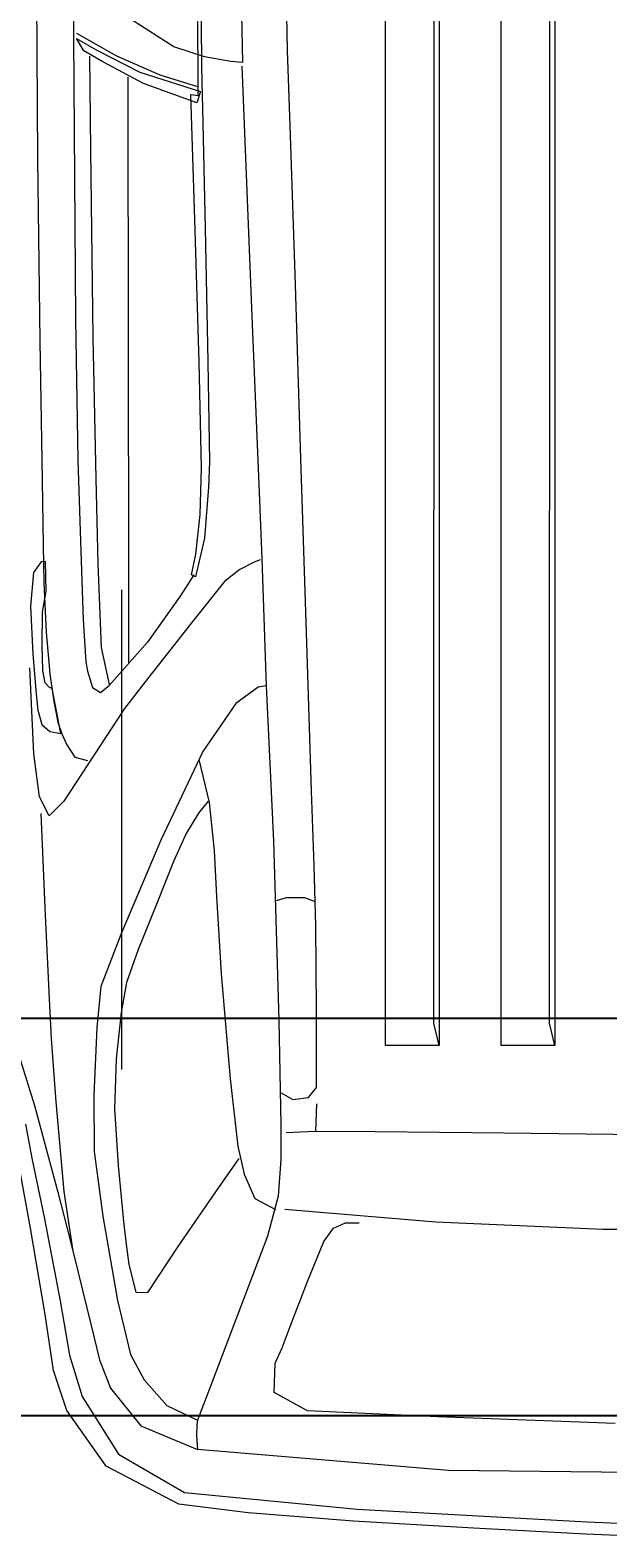
# Model space of a CAD drawing. Units: inches. Extents: x -5 to 482, y -460 to 66.
# Tile 4 of 31: x 52 to 66, y -389 to -351. Entities that reach past the tile are written whole.
import ezdxf

# ---------------------------------------------------------------- set-up
doc = ezdxf.new("R2010")
doc.units = ezdxf.units.IN
doc.header["$MEASUREMENT"] = 0
doc.layers.add('A-ANNO-DIMS', color=2, linetype='Continuous', lineweight=18)
doc.layers.add('A-EQPM-VEHI', color=8, linetype='Continuous', lineweight=13)
doc.styles.get("Standard").update_dxf_attribs({"font": 'arial.ttf'})
doc.dimstyles.get("Standard").update_dxf_attribs({"dimtxt": 0.18, "dimasz": 0.18, "dimexe": 0.18, "dimexo": 0.0625, "dimgap": 0.09, "dimtad": 0, "dimtih": 1, "dimtoh": 1, "dimdec": 0, "dimzin": 0, "dimdsep": 46, "dimlunit": 3, "dimtxsty": 'Standard', "dimcen": 0.09, "dimadec": 0, "dimazin": 0, "dimtfac": 1, "dimtdec": 0, "dimtofl": 0, "dimtmove": 0, "dimatfit": 3, "dimfxl": 1, "dimtolj": 1, "dimtzin": 0, "dimarcsym": 0})

# ---------------------------------------------------------------- blocks, each defined once
blk = doc.blocks.new('*D72')
at = {"layer": 'A-ANNO-DIMS', "color": 0, "lineweight": -2, "transparency": 16777216}
for p, q in [((144.314, -375.861), (-4.903, -375.861)), ((-4.723, -376.041), (-4.723, -380.679)), ((-4.723, -385.681), (-4.723, -381.043)), ((144.314, -385.861), (-4.903, -385.861))]:
    blk.add_line(p, q, dxfattribs=at)
at = {"layer": 'A-ANNO-DIMS', "color": 0, "transparency": 16777216}
for points in [[(-4.753, -376.041), (-4.693, -376.041), (-4.723, -375.861)], [(-4.753, -385.681), (-4.693, -385.681), (-4.723, -385.861)]]:
    blk.add_solid(points, dxfattribs=at)
at = {"layer": 'Defpoints', "color": 0, "transparency": 16777216}
for p in [(144.377, -375.861), (-4.723, -385.861), (144.377, -385.861)]:
    blk.add_point(p, dxfattribs=at)
at = {"layer": 'A-ANNO-DIMS', "color": 0, "transparency": 16777216, "insert": (-4.723, -380.861), "char_height": 0.18, "attachment_point": 5}
blk.add_mtext('\\A1;0\'-10"', dxfattribs=at)

msp = doc.modelspace()

# ---------------------------------------------------------------- linework, layer by layer
at = {"layer": 'A-EQPM-VEHI'}
for p, q in [((60.892, -376.546), (60.892, -341.062)), ((62.109, -375.982), (62.122, -341.174)), ((62.244, -341.062), (62.244, -376.546)), ((62.245, -341.062), (62.245, -376.546)), ((63.806, -376.546), (63.806, -341.062)), ((65.023, -375.982), (65.036, -341.174)), ((65.157, -341.062), (65.157, -376.546)), ((65.159, -341.062), (65.159, -376.546)), ((53.028, -348.051), (53.041, -351.173)), ((57.213, -347.914), (57.291, -351.814)), ((52.108, -349.325), (52.134, -354.234)), ((58.428, -351.511), (58.394, -349.773)), ((56.182, -352.643), (56.17, -350.375)), ((56.245, -350.247), (56.261, -351.733)), ((55.564, -351.42), (54.515, -350.745)), ((53.041, -351.173), (53.054, -353.537)), ((53.114, -351.078), (54.124, -351.644)), ((53.301, -351.524), (53.119, -351.212)), ((53.119, -351.212), (53.614, -351.498)), ((53.78, -351.798), (53.301, -351.524)), ((53.614, -351.498), (54.712, -352.059)), ((56.336, -351.673), (55.564, -351.42)), ((58.496, -353.407), (58.428, -351.511)), ((53.444, -351.654), (53.47, -354.014)), ((54.801, -352.339), (53.78, -351.798)), ((54.124, -351.644), (55.215, -352.124)), ((56.261, -351.733), (56.264, -351.884)), ((56.264, -351.884), (56.272, -352.31)), ((57.005, -351.787), (56.336, -351.673)), ((57.291, -351.814), (57.005, -351.787)), ((57.28, -351.903), (57.545, -358.611)), ((54.407, -352.175), (54.416, -359.209)), ((54.712, -352.059), (56.234, -352.546)), ((56.144, -352.824), (54.801, -352.339)), ((55.215, -352.124), (56.189, -352.422)), ((56.272, -352.31), (56.284, -352.966)), ((56.092, -355.767), (55.994, -352.617)), ((55.994, -352.617), (56.182, -352.643)), ((56.234, -352.546), (56.144, -352.824)), ((56.284, -352.966), (56.351, -355.986)), ((58.618, -357.135), (58.496, -353.407)), ((53.054, -353.537), (53.091, -358.267)), ((52.134, -354.234), (52.192, -358.825)), ((53.47, -354.014), (53.53, -358.735)), ((56.203, -359.353), (56.092, -355.767)), ((56.351, -355.986), (56.426, -359.336)), ((58.765, -361.777), (58.618, -357.135)), ((53.091, -358.267), (53.149, -361.818)), ((53.53, -358.735), (53.6, -362.282)), ((57.545, -358.611), (57.72, -362.834)), ((52.192, -358.825), (52.25, -362.326)), ((54.416, -359.209), (54.422, -364.236)), ((56.267, -362.008), (56.203, -359.353)), ((56.426, -359.336), (56.462, -361.858)), ((53.149, -361.818), (53.216, -363.856)), ((58.913, -366.416), (58.765, -361.777)), ((56.227, -363.182), (56.267, -362.008)), ((56.462, -361.858), (56.439, -362.497)), ((52.25, -362.326), (52.276, -363.967)), ((53.6, -362.282), (53.651, -364.423)), ((56.439, -362.497), (56.338, -363.779)), ((57.72, -362.834), (57.784, -364.303)), ((56.121, -364.183), (56.227, -363.182)), ((52.276, -363.967), (52.297, -364.9)), ((53.216, -363.856), (53.283, -365.835)), ((56.338, -363.779), (56.111, -364.753)), ((52.227, -364.379), (52.037, -364.646)), ((52.332, -364.363), (52.227, -364.379)), ((52.351, -365.116), (52.332, -364.363)), ((53.651, -364.423), (53.733, -366.529)), ((54.422, -364.236), (54.425, -366.922)), ((56.007, -364.701), (56.121, -364.183)), ((57.585, -364.386), (57.228, -364.565)), ((57.743, -364.328), (57.585, -364.386)), ((57.784, -364.303), (57.887, -367.491)), ((52.037, -364.646), (51.954, -365.489)), ((56.071, -364.706), (55.724, -365.243)), ((56.111, -364.753), (56.007, -364.701)), ((56.843, -364.874), (56.041, -365.865)), ((57.228, -364.565), (56.843, -364.874)), ((52.256, -365.643), (52.351, -365.116)), ((52.297, -364.9), (52.356, -366.146)), ((54.25, -365.078), (54.25, -377.149)), ((55.724, -365.243), (54.904, -366.396)), ((51.954, -365.489), (52.015, -366.701)), ((52.252, -366.46), (52.256, -365.643)), ((53.283, -365.835), (53.351, -366.889)), ((56.041, -365.865), (54.903, -367.319)), ((52.356, -366.146), (52.444, -367.191)), ((54.904, -366.396), (53.94, -367.483)), ((52.015, -366.701), (52.098, -367.695)), ((52.267, -367.107), (52.252, -366.46)), ((53.733, -366.529), (53.939, -367.459)), ((59.035, -370.135), (58.913, -366.416)), ((52.041, -369.206), (51.944, -367.039)), ((52.328, -367.416), (52.267, -367.107)), ((53.351, -366.889), (53.395, -367.126)), ((53.395, -367.126), (53.521, -367.535)), ((52.44, -367.54), (52.328, -367.416)), ((52.501, -367.563), (52.44, -367.54)), ((52.444, -367.191), (52.545, -367.889)), ((53.521, -367.535), (53.72, -367.661)), ((53.865, -367.548), (53.94, -367.483)), ((54.903, -367.319), (54.325, -368.064)), ((57.686, -367.529), (57.131, -367.936)), ((57.887, -367.491), (57.686, -367.529)), ((57.887, -367.491), (58.074, -371.406)), ((52.098, -367.695), (52.139, -368.106)), ((52.722, -368.694), (52.501, -367.563)), ((52.545, -367.889), (52.645, -368.408)), ((53.72, -367.661), (53.792, -367.608)), ((53.792, -367.608), (53.865, -367.548)), ((52.139, -368.106), (52.244, -368.469)), ((54.325, -368.064), (52.794, -370.398)), ((57.131, -367.936), (56.299, -369.146)), ((52.244, -368.469), (52.447, -368.643)), ((52.447, -368.643), (52.722, -368.694)), ((52.645, -368.408), (52.746, -368.702)), ((52.746, -368.702), (52.872, -368.979)), ((52.872, -368.979), (53.074, -369.292)), ((52.185, -370.291), (52.041, -369.206)), ((53.074, -369.292), (53.392, -369.371)), ((56.299, -369.146), (55.236, -371.377)), ((56.198, -369.349), (56.454, -370.43)), ((59.103, -372.018), (59.035, -370.135)), ((52.43, -370.768), (52.185, -370.291)), ((52.794, -370.398), (52.43, -370.768)), ((56.434, -370.396), (56.184, -370.7)), ((56.454, -370.43), (56.583, -371.646)), ((52.222, -370.71), (52.326, -373.268)), ((56.184, -370.7), (55.874, -371.207)), ((55.874, -371.207), (55.556, -371.916)), ((55.236, -371.377), (54.232, -373.751)), ((56.583, -371.646), (56.637, -372.795)), ((58.074, -371.406), (58.207, -375.907)), ((55.556, -371.916), (55.137, -372.967)), ((59.141, -373.534), (59.103, -372.018)), ((56.637, -372.795), (56.762, -374.739)), ((58.153, -372.896), (58.399, -372.817)), ((58.399, -372.817), (58.854, -372.821)), ((58.854, -372.821), (59.096, -372.915)), ((55.137, -372.967), (54.658, -374.154)), ((52.326, -373.268), (52.422, -375.192)), ((59.159, -375.649), (59.141, -373.534)), ((54.232, -373.751), (53.732, -375.058)), ((54.658, -374.154), (54.374, -374.957)), ((56.762, -374.739), (56.985, -377.382)), ((53.732, -375.058), (53.628, -376.091)), ((54.374, -374.957), (54.242, -375.713)), ((52.422, -375.192), (52.482, -376.376)), ((54.242, -375.713), (54.111, -376.881)), ((59.16, -377.601), (59.159, -375.649)), ((53.628, -376.091), (53.554, -377.799)), ((58.207, -375.907), (58.259, -378.538)), ((62.244, -376.546), (62.109, -375.982)), ((65.157, -376.546), (65.023, -375.982)), ((51.502, -376.274), (52.059, -378.05)), ((52.482, -376.376), (52.592, -377.962)), ((62.245, -376.546), (60.892, -376.546)), ((65.159, -376.546), (63.806, -376.546)), ((54.111, -376.881), (54.07, -378.133)), ((56.985, -377.382), (57.178, -379.079)), ((58.272, -377.731), (58.562, -377.906)), ((58.959, -377.85), (59.16, -377.601)), ((52.059, -378.05), (52.646, -380.231)), ((52.592, -377.962), (52.799, -380.217)), ((53.554, -377.799), (53.563, -379.214)), ((54.07, -378.133), (54.163, -379.56)), ((58.562, -377.906), (58.959, -377.85)), ((59.16, -378.014), (59.137, -378.707)), ((51.831, -378.52), (51.992, -379.38)), ((58.259, -378.538), (58.261, -379.415)), ((58.572, -378.732), (58.394, -378.741)), ((58.937, -378.716), (58.572, -378.732)), ((59.137, -378.707), (58.937, -378.716)), ((60.637, -378.714), (59.137, -378.707)), ((63.876, -378.752), (60.637, -378.714)), ((68.079, -378.796), (63.876, -378.752)), ((53.563, -379.214), (53.777, -380.837)), ((57.178, -379.079), (57.333, -379.783)), ((51.962, -381.14), (51.679, -379.625)), ((51.992, -379.38), (52.298, -380.859)), ((54.163, -379.56), (54.302, -380.973)), ((56.698, -380.116), (57.211, -379.383)), ((58.261, -379.415), (58.189, -380.33)), ((57.333, -379.783), (57.608, -380.39)), ((52.646, -380.231), (52.955, -381.444)), ((52.799, -380.217), (53.022, -381.714)), ((55.675, -381.6), (56.698, -380.116)), ((57.608, -380.39), (58.124, -380.666)), ((58.189, -380.33), (57.921, -381.342)), ((62.163, -380.985), (58.36, -380.666)), ((52.324, -383.315), (51.962, -381.14)), ((52.298, -380.859), (52.702, -382.964)), ((53.777, -380.837), (54.148, -382.962)), ((54.302, -380.973), (54.374, -381.612)), ((59.34, -381.477), (59.583, -381.139)), ((59.583, -381.139), (59.892, -381.007)), ((59.892, -381.007), (60.234, -381.003)), ((66.371, -381.169), (62.163, -380.985)), ((69.002, -381.173), (66.371, -381.169)), ((52.955, -381.444), (53.155, -382.253)), ((57.921, -381.342), (57.285, -383.021)), ((58.933, -382.484), (59.34, -381.477)), ((54.374, -381.612), (54.431, -382.053)), ((54.914, -382.761), (55.675, -381.6)), ((53.155, -382.253), (53.475, -383.551)), ((54.431, -382.053), (54.609, -382.749)), ((58.496, -383.612), (58.933, -382.484)), ((52.702, -382.964), (52.941, -384.33)), ((54.148, -382.962), (54.475, -384.315)), ((54.609, -382.749), (54.914, -382.761)), ((57.285, -383.021), (56.529, -385.008)), ((52.539, -384.717), (52.324, -383.315)), ((53.475, -383.551), (53.698, -384.45)), ((58.293, -384.146), (58.496, -383.612)), ((58.121, -384.535), (58.293, -384.146)), ((52.941, -384.33), (53.259, -385.373)), ((53.698, -384.45), (53.975, -385.163)), ((54.475, -384.315), (54.823, -384.953)), ((58.092, -385.277), (58.121, -384.535)), ((52.874, -385.729), (52.539, -384.717)), ((54.823, -384.953), (55.388, -385.598)), ((53.975, -385.163), (54.732, -386.109)), ((56.529, -385.008), (56.164, -385.966)), ((58.934, -385.734), (58.092, -385.277)), ((53.866, -387.126), (52.874, -385.729)), ((53.259, -385.373), (54.175, -386.827)), ((55.388, -385.598), (56.164, -385.966)), ((62.203, -385.884), (58.934, -385.734)), ((54.732, -386.109), (56.164, -386.71)), ((56.149, -386.084), (56.134, -386.367)), ((56.164, -385.966), (56.149, -386.084)), ((66.68, -386.057), (62.203, -385.884)), ((56.134, -386.367), (56.164, -386.71)), ((54.175, -386.827), (55.838, -387.789)), ((62.484, -387.232), (56.164, -386.71)), ((55.694, -388.083), (53.866, -387.126)), ((67.108, -387.283), (62.484, -387.232)), ((55.838, -387.789), (60.184, -388.207)), ((57.435, -388.302), (55.694, -388.083)), ((60.091, -388.508), (57.435, -388.302)), ((60.184, -388.207), (65.973, -388.525)), ((63.111, -388.69), (60.091, -388.508)), ((65.94, -388.834), (63.111, -388.69)), ((65.973, -388.525), (68.873, -388.652)), ((68.039, -388.93), (65.94, -388.834))]:
    msp.add_line(p, q, dxfattribs=at)

# ---------------------------------------------------------------- dimensions: what is measured, and where the dimension line sits
at = {"layer": 'A-ANNO-DIMS'}
dim = msp.add_linear_dim(base=(-4.723, -385.861), p1=(144.377, -375.861), p2=(144.377, -385.861), angle=90, dimstyle='Standard', override={"dimdec": 1, "dimlfac": 1, "dimrnd": 0, "dimzin": 1, "dimdsep": 46, "dimlunit": 4, "dimfrac": 2}, dxfattribs=at)
dim.commit()
dim.dimension.update_dxf_attribs({"geometry": '*D72', "text_midpoint": (-4.723, -380.861)})

doc.saveas('drawing.dxf')
